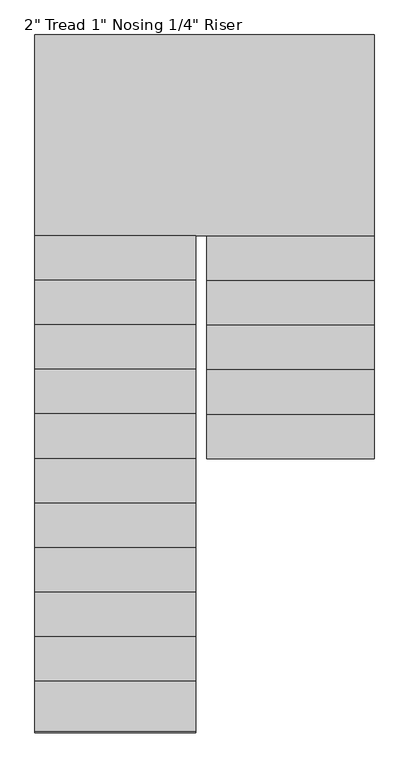
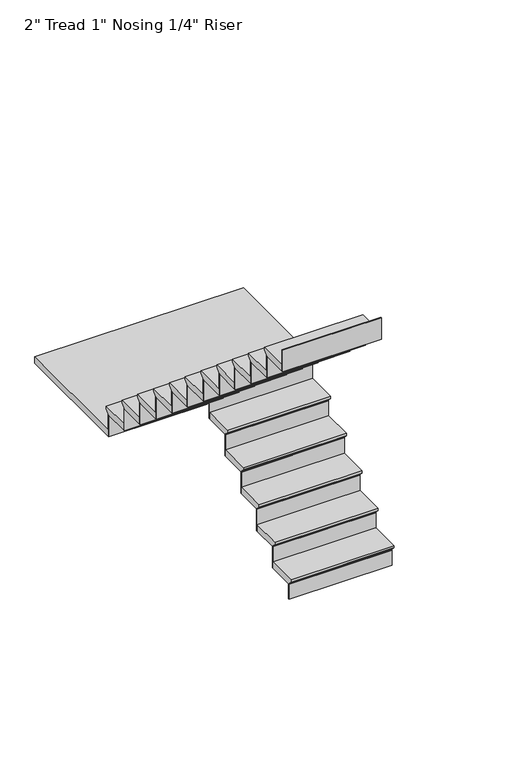
"""IFC4 building model written with IfcOpenShell, lengths in millimetres: stair flight geometry."""

from ifc_helpers import new_model, si_unit, origin, place, context, project, spatial, faceted_brep, source, transform, mapped, element, save


def stair_flight_9ad1fb7f(model_context):
    return source(origin(), model_context, "Body", "Brep", [
        faceted_brep([(-3749.597125, 2714.6319226, 15237.8833333), (-3749.597125, 2714.6319226, 15256.9333333), (-4512.2136682, 2714.6319226, 15256.9333333), (-4512.2136682, 2714.6319226, 15237.8833333), (-3749.597125, 2740.0319226, 15212.4833333), (-4512.2136682, 2740.0319226, 15212.4833333), (-3749.597125, 2943.2319226, 15256.9333333), (-4512.2136682, 2943.2319226, 15256.9333333), (-4512.2136682, 2740.0319226, 15206.1333333), (-4512.2136682, 2943.2319226, 15206.1333333), (-3749.597125, 2943.2319226, 15206.1333333), (-3749.597125, 2740.0319226, 15206.1333333)], [[[0, 1, 2, 3]], [[4, 0, 3, 5]], [[2, 1, 6, 7]], [[8, 9, 10, 11]], [[2, 7, 9, 8, 5, 3]], [[8, 11, 4, 5]], [[6, 1, 0, 4, 11, 10]], [[7, 6, 10, 9]]]),
        faceted_brep([(-3749.597125, 2740.0319226, 15206.1333333), (-3749.597125, 2740.0319226, 15087.6), (-3749.597125, 2746.3819226, 15087.6), (-3749.597125, 2746.3819226, 15206.1333333), (-4512.2136682, 2740.0319226, 15206.1333333), (-4512.2136682, 2746.3819226, 15206.1333333), (-4512.2136682, 2746.3819226, 15087.6), (-4512.2136682, 2740.0319226, 15087.6)], [[[0, 1, 2, 3]], [[4, 5, 6, 7]], [[1, 0, 4, 7]], [[2, 1, 7, 6]], [[3, 2, 6, 5]], [[0, 3, 5, 4]]]),
        faceted_brep([(-3749.597125, 2943.2319226, 15375.4666667), (-3749.597125, 2943.2319226, 15206.1333333), (-3749.597125, 2949.5819226, 15206.1333333), (-3749.597125, 2949.5819226, 15375.4666667), (-4512.2136682, 2943.2319226, 15375.4666667), (-4512.2136682, 2949.5819226, 15375.4666667), (-4512.2136682, 2949.5819226, 15206.1333333), (-4512.2136682, 2943.2319226, 15206.1333333)], [[[0, 1, 2, 3]], [[4, 5, 6, 7]], [[1, 0, 4, 7]], [[2, 1, 7, 6]], [[3, 2, 6, 5]], [[0, 3, 5, 4]]]),
        faceted_brep([(-4512.2136682, 2917.8319226, 15426.2666667), (-3749.597125, 2917.8319226, 15426.2666667), (-3749.597125, 3146.4319226, 15426.2666667), (-4512.2136682, 3146.4319226, 15426.2666667), (-4512.2136682, 2943.2319226, 15375.4666667), (-4512.2136682, 3146.4319226, 15375.4666667), (-3749.597125, 3146.4319226, 15375.4666667), (-3749.597125, 2943.2319226, 15375.4666667), (-4512.2136682, 2943.2319226, 15381.8166667), (-4512.2136682, 2917.8319226, 15407.2166667), (-3749.597125, 2943.2319226, 15381.8166667), (-3749.597125, 2917.8319226, 15407.2166667)], [[[0, 1, 2, 3]], [[4, 5, 6, 7]], [[0, 3, 5, 4, 8, 9]], [[4, 7, 10, 8]], [[2, 1, 11, 10, 7, 6]], [[3, 2, 6, 5]], [[11, 1, 0, 9]], [[10, 11, 9, 8]]]),
        faceted_brep([(-3749.597125, 3146.4319226, 15544.8), (-3749.597125, 3146.4319226, 15375.4666667), (-3749.597125, 3152.7819226, 15375.4666667), (-3749.597125, 3152.7819226, 15544.8), (-4512.2136682, 3146.4319226, 15544.8), (-4512.2136682, 3152.7819226, 15544.8), (-4512.2136682, 3152.7819226, 15375.4666667), (-4512.2136682, 3146.4319226, 15375.4666667)], [[[0, 1, 2, 3]], [[4, 5, 6, 7]], [[1, 0, 4, 7]], [[2, 1, 7, 6]], [[3, 2, 6, 5]], [[0, 3, 5, 4]]]),
        faceted_brep([(-4512.2136682, 3121.0319226, 15595.6), (-3749.597125, 3121.0319226, 15595.6), (-3749.597125, 3349.6319226, 15595.6), (-4512.2136682, 3349.6319226, 15595.6), (-4512.2136682, 3146.4319226, 15544.8), (-4512.2136682, 3349.6319226, 15544.8), (-3749.597125, 3349.6319226, 15544.8), (-3749.597125, 3146.4319226, 15544.8), (-4512.2136682, 3146.4319226, 15551.15), (-4512.2136682, 3121.0319226, 15576.55), (-3749.597125, 3146.4319226, 15551.15), (-3749.597125, 3121.0319226, 15576.55)], [[[0, 1, 2, 3]], [[4, 5, 6, 7]], [[0, 3, 5, 4, 8, 9]], [[4, 7, 10, 8]], [[2, 1, 11, 10, 7, 6]], [[3, 2, 6, 5]], [[11, 1, 0, 9]], [[10, 11, 9, 8]]]),
        faceted_brep([(-3749.597125, 3349.6319226, 15714.1333333), (-3749.597125, 3349.6319226, 15544.8), (-3749.597125, 3355.9819226, 15544.8), (-3749.597125, 3355.9819226, 15714.1333333), (-4512.2136682, 3349.6319226, 15714.1333333), (-4512.2136682, 3355.9819226, 15714.1333333), (-4512.2136682, 3355.9819226, 15544.8), (-4512.2136682, 3349.6319226, 15544.8)], [[[0, 1, 2, 3]], [[4, 5, 6, 7]], [[1, 0, 4, 7]], [[2, 1, 7, 6]], [[3, 2, 6, 5]], [[0, 3, 5, 4]]]),
        faceted_brep([(-4512.2136682, 3324.2319226, 15764.9333333), (-3749.597125, 3324.2319226, 15764.9333333), (-3749.597125, 3552.8319226, 15764.9333333), (-4512.2136682, 3552.8319226, 15764.9333333), (-4512.2136682, 3349.6319226, 15714.1333333), (-4512.2136682, 3552.8319226, 15714.1333333), (-3749.597125, 3552.8319226, 15714.1333333), (-3749.597125, 3349.6319226, 15714.1333333), (-4512.2136682, 3349.6319226, 15720.4833333), (-4512.2136682, 3324.2319226, 15745.8833333), (-3749.597125, 3349.6319226, 15720.4833333), (-3749.597125, 3324.2319226, 15745.8833333)], [[[0, 1, 2, 3]], [[4, 5, 6, 7]], [[0, 3, 5, 4, 8, 9]], [[4, 7, 10, 8]], [[2, 1, 11, 10, 7, 6]], [[3, 2, 6, 5]], [[11, 1, 0, 9]], [[10, 11, 9, 8]]]),
        faceted_brep([(-3749.597125, 3552.8319226, 15883.4666667), (-3749.597125, 3552.8319226, 15714.1333333), (-3749.597125, 3559.1819226, 15714.1333333), (-3749.597125, 3559.1819226, 15883.4666667), (-4512.2136682, 3552.8319226, 15883.4666667), (-4512.2136682, 3559.1819226, 15883.4666667), (-4512.2136682, 3559.1819226, 15714.1333333), (-4512.2136682, 3552.8319226, 15714.1333333)], [[[0, 1, 2, 3]], [[4, 5, 6, 7]], [[1, 0, 4, 7]], [[2, 1, 7, 6]], [[3, 2, 6, 5]], [[0, 3, 5, 4]]]),
        faceted_brep([(-4512.2136682, 3527.4319226, 15934.2666667), (-3749.597125, 3527.4319226, 15934.2666667), (-3749.597125, 3756.0319226, 15934.2666667), (-4512.2136682, 3756.0319226, 15934.2666667), (-4512.2136682, 3552.8319226, 15883.4666667), (-4512.2136682, 3756.0319226, 15883.4666667), (-3749.597125, 3756.0319226, 15883.4666667), (-3749.597125, 3552.8319226, 15883.4666667), (-4512.2136682, 3552.8319226, 15889.8166667), (-4512.2136682, 3527.4319226, 15915.2166667), (-3749.597125, 3552.8319226, 15889.8166667), (-3749.597125, 3527.4319226, 15915.2166667)], [[[0, 1, 2, 3]], [[4, 5, 6, 7]], [[0, 3, 5, 4, 8, 9]], [[4, 7, 10, 8]], [[2, 1, 11, 10, 7, 6]], [[3, 2, 6, 5]], [[11, 1, 0, 9]], [[10, 11, 9, 8]]]),
        faceted_brep([(-3749.597125, 3756.0319226, 16052.8), (-3749.597125, 3756.0319226, 15883.4666667), (-3749.597125, 3762.3819226, 15883.4666667), (-3749.597125, 3762.3819226, 16052.8), (-4512.2136682, 3756.0319226, 16052.8), (-4512.2136682, 3762.3819226, 16052.8), (-4512.2136682, 3762.3819226, 15883.4666667), (-4512.2136682, 3756.0319226, 15883.4666667)], [[[0, 1, 2, 3]], [[4, 5, 6, 7]], [[1, 0, 4, 7]], [[2, 1, 7, 6]], [[3, 2, 6, 5]], [[0, 3, 5, 4]]]),
        faceted_brep([(-4563.0136682, 3705.2319226, 16103.6), (-4563.0136682, 3730.6319226, 16103.6), (-3749.597125, 3730.6319226, 16103.6), (-3749.597125, 4645.0319226, 16103.6), (-5295.0246464, 4645.0319226, 16103.6), (-5295.0246464, 3705.2319226, 16103.6), (-4563.0136682, 3730.6319226, 16052.8), (-4563.0136682, 3705.2319226, 16052.8), (-5295.0246464, 3705.2319226, 16052.8), (-5295.0246464, 4645.0319226, 16052.8), (-3749.597125, 4645.0319226, 16052.8), (-3749.597125, 3756.0319226, 16052.8), (-4512.2136682, 3756.0319226, 16052.8), (-4512.2136682, 3730.6319226, 16052.8), (-4512.2136682, 3730.6319226, 16084.55), (-3749.597125, 3730.6319226, 16084.55), (-4512.2136682, 3756.0319226, 16059.15), (-3749.597125, 3756.0319226, 16059.15)], [[[0, 1, 2, 3, 4, 5]], [[6, 7, 8, 9, 10, 11, 12, 13]], [[1, 0, 7, 6]], [[2, 1, 6, 13, 14, 15]], [[13, 12, 16, 14]], [[12, 11, 17, 16]], [[3, 2, 15, 17, 11, 10]], [[4, 3, 10, 9]], [[5, 4, 9, 8]], [[0, 5, 8, 7]], [[17, 15, 14, 16]]]),
        faceted_brep([(-5295.0246464, 3705.2319226, 16222.1333333), (-5295.0246464, 3705.2319226, 16052.8), (-5295.0246464, 3698.8819226, 16052.8), (-5295.0246464, 3698.8819226, 16222.1333333), (-4563.0136682, 3705.2319226, 16222.1333333), (-4563.0136682, 3698.8819226, 16222.1333333), (-4563.0136682, 3698.8819226, 16052.8), (-4563.0136682, 3705.2319226, 16052.8)], [[[0, 1, 2, 3]], [[4, 5, 6, 7]], [[1, 0, 4, 7]], [[2, 1, 7, 6]], [[3, 2, 6, 5]], [[0, 3, 5, 4]]]),
        faceted_brep([(-4563.0136682, 3730.6319226, 16272.9333333), (-5295.0246464, 3730.6319226, 16272.9333333), (-5295.0246464, 3502.0319226, 16272.9333333), (-4563.0136682, 3502.0319226, 16272.9333333), (-4563.0136682, 3705.2319226, 16222.1333333), (-4563.0136682, 3502.0319226, 16222.1333333), (-5295.0246464, 3502.0319226, 16222.1333333), (-5295.0246464, 3705.2319226, 16222.1333333), (-4563.0136682, 3705.2319226, 16228.4833333), (-4563.0136682, 3730.6319226, 16253.8833333), (-5295.0246464, 3705.2319226, 16228.4833333), (-5295.0246464, 3730.6319226, 16253.8833333)], [[[0, 1, 2, 3]], [[4, 5, 6, 7]], [[0, 3, 5, 4, 8, 9]], [[4, 7, 10, 8]], [[2, 1, 11, 10, 7, 6]], [[3, 2, 6, 5]], [[11, 1, 0, 9]], [[10, 11, 9, 8]]]),
        faceted_brep([(-5295.0246464, 3502.0319226, 16391.4666667), (-5295.0246464, 3502.0319226, 16222.1333333), (-5295.0246464, 3495.6819226, 16222.1333333), (-5295.0246464, 3495.6819226, 16391.4666667), (-4563.0136682, 3502.0319226, 16391.4666667), (-4563.0136682, 3495.6819226, 16391.4666667), (-4563.0136682, 3495.6819226, 16222.1333333), (-4563.0136682, 3502.0319226, 16222.1333333)], [[[0, 1, 2, 3]], [[4, 5, 6, 7]], [[1, 0, 4, 7]], [[2, 1, 7, 6]], [[3, 2, 6, 5]], [[0, 3, 5, 4]]]),
        faceted_brep([(-4563.0136682, 3527.4319226, 16442.2666667), (-5295.0246464, 3527.4319226, 16442.2666667), (-5295.0246464, 3298.8319226, 16442.2666667), (-4563.0136682, 3298.8319226, 16442.2666667), (-4563.0136682, 3502.0319226, 16391.4666667), (-4563.0136682, 3298.8319226, 16391.4666667), (-5295.0246464, 3298.8319226, 16391.4666667), (-5295.0246464, 3502.0319226, 16391.4666667), (-4563.0136682, 3502.0319226, 16397.8166667), (-4563.0136682, 3527.4319226, 16423.2166667), (-5295.0246464, 3502.0319226, 16397.8166667), (-5295.0246464, 3527.4319226, 16423.2166667)], [[[0, 1, 2, 3]], [[4, 5, 6, 7]], [[0, 3, 5, 4, 8, 9]], [[4, 7, 10, 8]], [[2, 1, 11, 10, 7, 6]], [[3, 2, 6, 5]], [[11, 1, 0, 9]], [[10, 11, 9, 8]]]),
        faceted_brep([(-5295.0246464, 3298.8319226, 16560.8), (-5295.0246464, 3298.8319226, 16391.4666667), (-5295.0246464, 3292.4819226, 16391.4666667), (-5295.0246464, 3292.4819226, 16560.8), (-4563.0136682, 3298.8319226, 16560.8), (-4563.0136682, 3292.4819226, 16560.8), (-4563.0136682, 3292.4819226, 16391.4666667), (-4563.0136682, 3298.8319226, 16391.4666667)], [[[0, 1, 2, 3]], [[4, 5, 6, 7]], [[1, 0, 4, 7]], [[2, 1, 7, 6]], [[3, 2, 6, 5]], [[0, 3, 5, 4]]]),
        faceted_brep([(-4563.0136682, 3324.2319226, 16611.6), (-5295.0246464, 3324.2319226, 16611.6), (-5295.0246464, 3095.6319226, 16611.6), (-4563.0136682, 3095.6319226, 16611.6), (-4563.0136682, 3298.8319226, 16560.8), (-4563.0136682, 3095.6319226, 16560.8), (-5295.0246464, 3095.6319226, 16560.8), (-5295.0246464, 3298.8319226, 16560.8), (-4563.0136682, 3298.8319226, 16567.15), (-4563.0136682, 3324.2319226, 16592.55), (-5295.0246464, 3298.8319226, 16567.15), (-5295.0246464, 3324.2319226, 16592.55)], [[[0, 1, 2, 3]], [[4, 5, 6, 7]], [[0, 3, 5, 4, 8, 9]], [[4, 7, 10, 8]], [[2, 1, 11, 10, 7, 6]], [[3, 2, 6, 5]], [[11, 1, 0, 9]], [[10, 11, 9, 8]]]),
        faceted_brep([(-5295.0246464, 3095.6319226, 16730.1333333), (-5295.0246464, 3095.6319226, 16560.8), (-5295.0246464, 3089.2819226, 16560.8), (-5295.0246464, 3089.2819226, 16730.1333333), (-4563.0136682, 3095.6319226, 16730.1333333), (-4563.0136682, 3089.2819226, 16730.1333333), (-4563.0136682, 3089.2819226, 16560.8), (-4563.0136682, 3095.6319226, 16560.8)], [[[0, 1, 2, 3]], [[4, 5, 6, 7]], [[1, 0, 4, 7]], [[2, 1, 7, 6]], [[3, 2, 6, 5]], [[0, 3, 5, 4]]]),
        faceted_brep([(-4563.0136682, 3121.0319226, 16780.9333333), (-5295.0246464, 3121.0319226, 16780.9333333), (-5295.0246464, 2892.4319226, 16780.9333333), (-4563.0136682, 2892.4319226, 16780.9333333), (-4563.0136682, 3095.6319226, 16730.1333333), (-4563.0136682, 2892.4319226, 16730.1333333), (-5295.0246464, 2892.4319226, 16730.1333333), (-5295.0246464, 3095.6319226, 16730.1333333), (-4563.0136682, 3095.6319226, 16736.4833333), (-4563.0136682, 3121.0319226, 16761.8833333), (-5295.0246464, 3095.6319226, 16736.4833333), (-5295.0246464, 3121.0319226, 16761.8833333)], [[[0, 1, 2, 3]], [[4, 5, 6, 7]], [[0, 3, 5, 4, 8, 9]], [[4, 7, 10, 8]], [[2, 1, 11, 10, 7, 6]], [[3, 2, 6, 5]], [[11, 1, 0, 9]], [[10, 11, 9, 8]]]),
        faceted_brep([(-5295.0246464, 2892.4319226, 16899.4666667), (-5295.0246464, 2892.4319226, 16730.1333333), (-5295.0246464, 2886.0819226, 16730.1333333), (-5295.0246464, 2886.0819226, 16899.4666667), (-4563.0136682, 2892.4319226, 16899.4666667), (-4563.0136682, 2886.0819226, 16899.4666667), (-4563.0136682, 2886.0819226, 16730.1333333), (-4563.0136682, 2892.4319226, 16730.1333333)], [[[0, 1, 2, 3]], [[4, 5, 6, 7]], [[1, 0, 4, 7]], [[2, 1, 7, 6]], [[3, 2, 6, 5]], [[0, 3, 5, 4]]]),
        faceted_brep([(-4563.0136682, 2917.8319226, 16950.2666667), (-5295.0246464, 2917.8319226, 16950.2666667), (-5295.0246464, 2689.2319226, 16950.2666667), (-4563.0136682, 2689.2319226, 16950.2666667), (-4563.0136682, 2892.4319226, 16899.4666667), (-4563.0136682, 2689.2319226, 16899.4666667), (-5295.0246464, 2689.2319226, 16899.4666667), (-5295.0246464, 2892.4319226, 16899.4666667), (-4563.0136682, 2892.4319226, 16905.8166667), (-4563.0136682, 2917.8319226, 16931.2166667), (-5295.0246464, 2892.4319226, 16905.8166667), (-5295.0246464, 2917.8319226, 16931.2166667)], [[[0, 1, 2, 3]], [[4, 5, 6, 7]], [[0, 3, 5, 4, 8, 9]], [[4, 7, 10, 8]], [[2, 1, 11, 10, 7, 6]], [[3, 2, 6, 5]], [[11, 1, 0, 9]], [[10, 11, 9, 8]]]),
        faceted_brep([(-5295.0246464, 2689.2319226, 17068.8), (-5295.0246464, 2689.2319226, 16899.4666667), (-5295.0246464, 2682.8819226, 16899.4666667), (-5295.0246464, 2682.8819226, 17068.8), (-4563.0136682, 2689.2319226, 17068.8), (-4563.0136682, 2682.8819226, 17068.8), (-4563.0136682, 2682.8819226, 16899.4666667), (-4563.0136682, 2689.2319226, 16899.4666667)], [[[0, 1, 2, 3]], [[4, 5, 6, 7]], [[1, 0, 4, 7]], [[2, 1, 7, 6]], [[3, 2, 6, 5]], [[0, 3, 5, 4]]]),
        faceted_brep([(-4563.0136682, 2714.6319226, 17119.6), (-5295.0246464, 2714.6319226, 17119.6), (-5295.0246464, 2486.0319226, 17119.6), (-4563.0136682, 2486.0319226, 17119.6), (-4563.0136682, 2689.2319226, 17068.8), (-4563.0136682, 2486.0319226, 17068.8), (-5295.0246464, 2486.0319226, 17068.8), (-5295.0246464, 2689.2319226, 17068.8), (-4563.0136682, 2689.2319226, 17075.15), (-4563.0136682, 2714.6319226, 17100.55), (-5295.0246464, 2689.2319226, 17075.15), (-5295.0246464, 2714.6319226, 17100.55)], [[[0, 1, 2, 3]], [[4, 5, 6, 7]], [[0, 3, 5, 4, 8, 9]], [[4, 7, 10, 8]], [[2, 1, 11, 10, 7, 6]], [[3, 2, 6, 5]], [[11, 1, 0, 9]], [[10, 11, 9, 8]]]),
        faceted_brep([(-5295.0246464, 2486.0319226, 17238.1333333), (-5295.0246464, 2486.0319226, 17068.8), (-5295.0246464, 2479.6819226, 17068.8), (-5295.0246464, 2479.6819226, 17238.1333333), (-4563.0136682, 2486.0319226, 17238.1333333), (-4563.0136682, 2479.6819226, 17238.1333333), (-4563.0136682, 2479.6819226, 17068.8), (-4563.0136682, 2486.0319226, 17068.8)], [[[0, 1, 2, 3]], [[4, 5, 6, 7]], [[1, 0, 4, 7]], [[2, 1, 7, 6]], [[3, 2, 6, 5]], [[0, 3, 5, 4]]]),
        faceted_brep([(-4563.0136682, 2511.4319226, 17288.9333333), (-5295.0246464, 2511.4319226, 17288.9333333), (-5295.0246464, 2282.8319226, 17288.9333333), (-4563.0136682, 2282.8319226, 17288.9333333), (-4563.0136682, 2486.0319226, 17238.1333333), (-4563.0136682, 2282.8319226, 17238.1333333), (-5295.0246464, 2282.8319226, 17238.1333333), (-5295.0246464, 2486.0319226, 17238.1333333), (-4563.0136682, 2486.0319226, 17244.4833333), (-4563.0136682, 2511.4319226, 17269.8833333), (-5295.0246464, 2486.0319226, 17244.4833333), (-5295.0246464, 2511.4319226, 17269.8833333)], [[[0, 1, 2, 3]], [[4, 5, 6, 7]], [[0, 3, 5, 4, 8, 9]], [[4, 7, 10, 8]], [[2, 1, 11, 10, 7, 6]], [[3, 2, 6, 5]], [[11, 1, 0, 9]], [[10, 11, 9, 8]]]),
        faceted_brep([(-5295.0246464, 2282.8319226, 17407.4666667), (-5295.0246464, 2282.8319226, 17238.1333333), (-5295.0246464, 2276.4819226, 17238.1333333), (-5295.0246464, 2276.4819226, 17407.4666667), (-4563.0136682, 2282.8319226, 17407.4666667), (-4563.0136682, 2276.4819226, 17407.4666667), (-4563.0136682, 2276.4819226, 17238.1333333), (-4563.0136682, 2282.8319226, 17238.1333333)], [[[0, 1, 2, 3]], [[4, 5, 6, 7]], [[1, 0, 4, 7]], [[2, 1, 7, 6]], [[3, 2, 6, 5]], [[0, 3, 5, 4]]]),
        faceted_brep([(-4563.0136682, 2308.2319226, 17458.2666667), (-5295.0246464, 2308.2319226, 17458.2666667), (-5295.0246464, 2079.6319226, 17458.2666667), (-4563.0136682, 2079.6319226, 17458.2666667), (-4563.0136682, 2282.8319226, 17407.4666667), (-4563.0136682, 2079.6319226, 17407.4666667), (-5295.0246464, 2079.6319226, 17407.4666667), (-5295.0246464, 2282.8319226, 17407.4666667), (-4563.0136682, 2282.8319226, 17413.8166667), (-4563.0136682, 2308.2319226, 17439.2166667), (-5295.0246464, 2282.8319226, 17413.8166667), (-5295.0246464, 2308.2319226, 17439.2166667)], [[[0, 1, 2, 3]], [[4, 5, 6, 7]], [[0, 3, 5, 4, 8, 9]], [[4, 7, 10, 8]], [[2, 1, 11, 10, 7, 6]], [[3, 2, 6, 5]], [[11, 1, 0, 9]], [[10, 11, 9, 8]]]),
        faceted_brep([(-5295.0246464, 2079.6319226, 17576.8), (-5295.0246464, 2079.6319226, 17407.4666667), (-5295.0246464, 2073.2819226, 17407.4666667), (-5295.0246464, 2073.2819226, 17576.8), (-4563.0136682, 2079.6319226, 17576.8), (-4563.0136682, 2073.2819226, 17576.8), (-4563.0136682, 2073.2819226, 17407.4666667), (-4563.0136682, 2079.6319226, 17407.4666667)], [[[0, 1, 2, 3]], [[4, 5, 6, 7]], [[1, 0, 4, 7]], [[2, 1, 7, 6]], [[3, 2, 6, 5]], [[0, 3, 5, 4]]]),
        faceted_brep([(-4563.0136682, 2105.0319226, 17627.6), (-5295.0246464, 2105.0319226, 17627.6), (-5295.0246464, 1876.4319226, 17627.6), (-4563.0136682, 1876.4319226, 17627.6), (-4563.0136682, 2079.6319226, 17576.8), (-4563.0136682, 1876.4319226, 17576.8), (-5295.0246464, 1876.4319226, 17576.8), (-5295.0246464, 2079.6319226, 17576.8), (-4563.0136682, 2079.6319226, 17583.15), (-4563.0136682, 2105.0319226, 17608.55), (-5295.0246464, 2079.6319226, 17583.15), (-5295.0246464, 2105.0319226, 17608.55)], [[[0, 1, 2, 3]], [[4, 5, 6, 7]], [[0, 3, 5, 4, 8, 9]], [[4, 7, 10, 8]], [[2, 1, 11, 10, 7, 6]], [[3, 2, 6, 5]], [[11, 1, 0, 9]], [[10, 11, 9, 8]]]),
        faceted_brep([(-5295.0246464, 1876.4319226, 17746.1333333), (-5295.0246464, 1876.4319226, 17576.8), (-5295.0246464, 1870.0819226, 17576.8), (-5295.0246464, 1870.0819226, 17746.1333333), (-4563.0136682, 1876.4319226, 17746.1333333), (-4563.0136682, 1870.0819226, 17746.1333333), (-4563.0136682, 1870.0819226, 17576.8), (-4563.0136682, 1876.4319226, 17576.8)], [[[0, 1, 2, 3]], [[4, 5, 6, 7]], [[1, 0, 4, 7]], [[2, 1, 7, 6]], [[3, 2, 6, 5]], [[0, 3, 5, 4]]]),
        faceted_brep([(-4563.0136682, 1901.8319226, 17796.9333333), (-5295.0246464, 1901.8319226, 17796.9333333), (-5295.0246464, 1673.2319226, 17796.9333333), (-4563.0136682, 1673.2319226, 17796.9333333), (-4563.0136682, 1876.4319226, 17746.1333333), (-4563.0136682, 1673.2319226, 17746.1333333), (-5295.0246464, 1673.2319226, 17746.1333333), (-5295.0246464, 1876.4319226, 17746.1333333), (-4563.0136682, 1876.4319226, 17752.4833333), (-4563.0136682, 1901.8319226, 17777.8833333), (-5295.0246464, 1876.4319226, 17752.4833333), (-5295.0246464, 1901.8319226, 17777.8833333)], [[[0, 1, 2, 3]], [[4, 5, 6, 7]], [[0, 3, 5, 4, 8, 9]], [[4, 7, 10, 8]], [[2, 1, 11, 10, 7, 6]], [[3, 2, 6, 5]], [[11, 1, 0, 9]], [[10, 11, 9, 8]]]),
        faceted_brep([(-5295.0246464, 1673.2319226, 17915.4666667), (-5295.0246464, 1673.2319226, 17746.1333333), (-5295.0246464, 1666.8819226, 17746.1333333), (-5295.0246464, 1666.8819226, 17915.4666667), (-4563.0136682, 1673.2319226, 17915.4666667), (-4563.0136682, 1666.8819226, 17915.4666667), (-4563.0136682, 1666.8819226, 17746.1333333), (-4563.0136682, 1673.2319226, 17746.1333333)], [[[0, 1, 2, 3]], [[4, 5, 6, 7]], [[1, 0, 4, 7]], [[2, 1, 7, 6]], [[3, 2, 6, 5]], [[0, 3, 5, 4]]]),
        faceted_brep([(-4563.0136682, 1698.6319226, 17966.2666667), (-5295.0246464, 1698.6319226, 17966.2666667), (-5295.0246464, 1470.0319226, 17966.2666667), (-4563.0136682, 1470.0319226, 17966.2666667), (-4563.0136682, 1673.2319226, 17915.4666667), (-4563.0136682, 1470.0319226, 17915.4666667), (-5295.0246464, 1470.0319226, 17915.4666667), (-5295.0246464, 1673.2319226, 17915.4666667), (-4563.0136682, 1673.2319226, 17921.8166667), (-4563.0136682, 1698.6319226, 17947.2166667), (-5295.0246464, 1673.2319226, 17921.8166667), (-5295.0246464, 1698.6319226, 17947.2166667)], [[[0, 1, 2, 3]], [[4, 5, 6, 7]], [[0, 3, 5, 4, 8, 9]], [[4, 7, 10, 8]], [[2, 1, 11, 10, 7, 6]], [[3, 2, 6, 5]], [[11, 1, 0, 9]], [[10, 11, 9, 8]]]),
        faceted_brep([(-5295.0246464, 1470.0319226, 18084.8), (-5295.0246464, 1470.0319226, 17915.4666667), (-5295.0246464, 1463.6819226, 17915.4666667), (-5295.0246464, 1463.6819226, 18084.8), (-4563.0136682, 1470.0319226, 18084.8), (-4563.0136682, 1463.6819226, 18084.8), (-4563.0136682, 1463.6819226, 17915.4666667), (-4563.0136682, 1470.0319226, 17915.4666667)], [[[0, 1, 2, 3]], [[4, 5, 6, 7]], [[1, 0, 4, 7]], [[2, 1, 7, 6]], [[3, 2, 6, 5]], [[0, 3, 5, 4]]]),
    ])


if __name__ == "__main__":
    model = new_model("IFC4")
    model_context = context("Model", 3, world=origin())
    ifc_project = project(units=[si_unit("LENGTHUNIT", "METRE", prefix="MILLI")], contexts=[model_context])
    site = spatial("IfcSite", under=ifc_project)
    building = spatial("IfcBuilding", under=site)
    placement = place(None, origin())
    stair_flight_shape = stair_flight_9ad1fb7f(model_context)
    element("IfcStairFlight", 1, ObjectType="2\" Tread 1\" Nosing 1/4\" Riser", at=placement, inside=building, context=model_context, shape_type="MappedRepresentation", body=[
        mapped(stair_flight_shape, transform((0.0, 0.0, 0.0), x_axis=(1.0, 0.0, 0.0), y_axis=(0.0, 1.0, 0.0), z_axis=(0.0, 0.0, 1.0))),
    ])
    save(model, "model.ifc")
